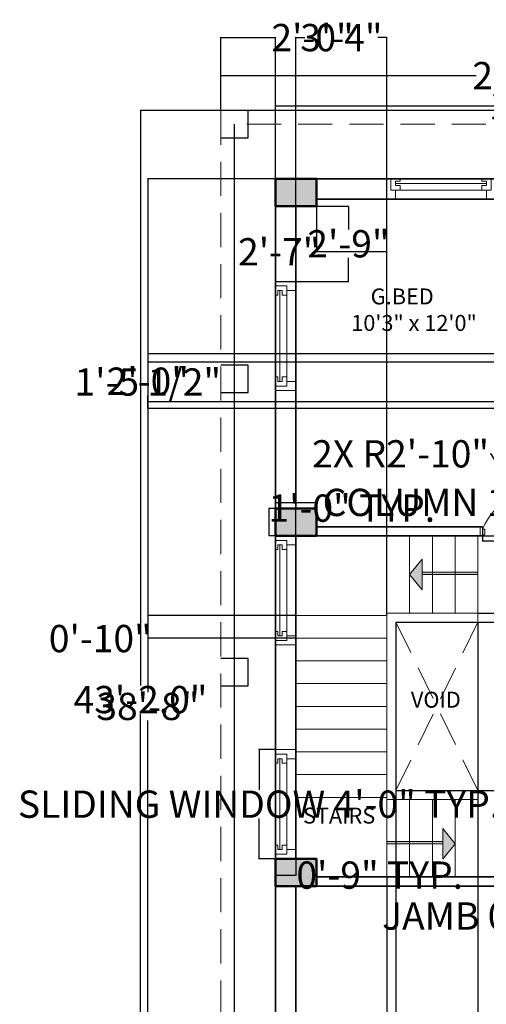
# Model space of a CAD drawing. Units: inches. Extents: x 1063 to 2718, y 423 to 1923.
# Tile 2 of 7: x 1063 to 1268, y 692 to 1125. Entities that reach past the tile are written whole.
import ezdxf

# ---------------------------------------------------------------- set-up
doc = ezdxf.new("R2010")
doc.units = ezdxf.units.IN
doc.header["$LTSCALE"] = 6
doc.header["$MEASUREMENT"] = 0
doc.linetypes.add('HIDDEN', pattern=[0.375, 0.25, -0.125])
for name, color, linetype, lineweight in [('A-ANNO-DIMS', 2, 'Continuous', 18), ('A-ANNO-SYMB', 4, 'Continuous', 18), ('A-ANNO-SYMB-PATT', 7, 'Continuous', 13), ('A-AREA-IDEN', 7, 'Continuous', 18), ('A-COLS', 7, 'Continuous', 50), ('A-COLS-PATT', 252, 'Continuous', 13), ('A-DOOR', 2, 'Continuous', 18), ('A-FLOR-STRS', 7, 'Continuous', 18), ('A-FLOR-STRS-HIDN', 7, 'HIDDEN', 13), ('A-GLAZ', 4, 'Continuous', 18), ('A-WALL', 7, 'Continuous', 35), ('C-PROP', 7, 'Continuous', 25), ('C-PROP-HIDN', 7, 'HIDDEN', 18)]:
    doc.layers.add(name, color=color, linetype=linetype, lineweight=lineweight)
doc.styles.get("Standard").update_dxf_attribs({"font": 'arial.ttf'})
doc.dimstyles.get("Standard").update_dxf_attribs({"dimtxt": 12, "dimasz": 0.18, "dimexe": 0.18, "dimexo": 0.0625, "dimgap": 0.09, "dimtad": 0, "dimtih": 1, "dimtoh": 1, "dimdec": 1, "dimzin": 0, "dimdsep": 46, "dimlunit": 3, "dimtxsty": 'Standard', "dimcen": 0.09, "dimadec": 0, "dimazin": 0, "dimtfac": 1, "dimtdec": 1, "dimtofl": 0, "dimtmove": 0, "dimatfit": 3, "dimfxl": 1, "dimtolj": 1, "dimtzin": 0, "dimarcsym": 0})

# ---------------------------------------------------------------- blocks, each defined once
blk = doc.blocks.new('*D1')
at = {"layer": 'A-ANNO-DIMS', "color": 0, "lineweight": -2, "ltscale": 6, "transparency": 16777216}
for p, q in [((1150.86, 1085.12), (1115.44, 1085.12)), ((1115.62, 1084.94), (1115.62, 832.34)), ((1115.62, 567.3), (1115.62, 819.9)), ((1150.86, 567.12), (1115.44, 567.12))]:
    blk.add_line(p, q, dxfattribs=at)
at = {"layer": 'A-ANNO-DIMS', "color": 0, "ltscale": 6, "transparency": 16777216}
for points in [[(1115.59, 1084.94), (1115.65, 1084.94), (1115.62, 1085.12)], [(1115.59, 567.3), (1115.65, 567.3), (1115.62, 567.12)]]:
    blk.add_solid(points, dxfattribs=at)
at = {"layer": 'Defpoints', "color": 0, "ltscale": 6, "transparency": 16777216}
for p in [(1115.62, 1085.12), (1150.93, 1085.12), (1150.93, 567.12)]:
    blk.add_point(p, dxfattribs=at)
at = {"layer": 'A-ANNO-DIMS', "color": 0, "ltscale": 6, "transparency": 16777216, "insert": (1115.62, 826.12), "char_height": 12, "attachment_point": 5}
blk.add_mtext('\\A1;43\'-2.0"', dxfattribs=at)
blk = doc.blocks.new('*D6')
at = {"layer": 'A-ANNO-DIMS', "color": 0, "lineweight": -2, "ltscale": 6, "transparency": 16777216}
for p, q in [((1150.93, 1085.18), (1150.93, 1100.66)), ((1151.11, 1100.48), (1263.13, 1100.48)), ((1430.75, 1100.48), (1318.72, 1100.48)), ((1430.93, 1085.18), (1430.93, 1100.66))]:
    blk.add_line(p, q, dxfattribs=at)
at = {"layer": 'A-ANNO-DIMS', "color": 0, "ltscale": 6, "transparency": 16777216}
for points in [[(1151.11, 1100.51), (1151.11, 1100.45), (1150.93, 1100.48)], [(1430.75, 1100.51), (1430.75, 1100.45), (1430.93, 1100.48)]]:
    blk.add_solid(points, dxfattribs=at)
at = {"layer": 'Defpoints', "color": 0, "ltscale": 6, "transparency": 16777216}
for p in [(1430.93, 1100.48), (1150.93, 1085.12), (1430.93, 1085.12)]:
    blk.add_point(p, dxfattribs=at)
at = {"layer": 'A-ANNO-DIMS', "color": 0, "ltscale": 6, "transparency": 16777216, "insert": (1290.93, 1100.48), "char_height": 12, "attachment_point": 5}
blk.add_mtext('\\A1;23\'-4.0"', dxfattribs=at)
blk = doc.blocks.new('WIN-48-SLIDING')
at = {"ltscale": 6}
for p, q in [((0, 9), (4, 9)), ((4, 9), (4, 5)), ((48, 9), (44, 9)), ((44, 9), (44, 5)), ((4, 5), (2, 5)), ((2, 5), (2, 0)), ((4, 5), (44, 5)), ((4, 5), (6, 5)), ((6, 5), (6, 3)), ((44, 5), (42, 5)), ((42, 5), (42, 3)), ((44, 5), (46, 5)), ((46, 5), (46, 0)), ((6, 3), (4, 3)), ((4, 3), (4, 1)), ((4, 2), (44, 2)), ((4, 1), (6, 1)), ((6, 1), (6, 0)), ((42, 3), (44, 3)), ((44, 1), (42, 1)), ((42, 1), (42, 0)), ((44, 3), (44, 1)), ((48, 0), (0, 0)), ((2, 0), (46, 0))]:
    blk.add_line(p, q, dxfattribs=at)
blk.add_lwpolyline([(48, 0), (48, 9), (0, 9), (0, 0)], dxfattribs=at)
blk = doc.blocks.new('DOOR-JAMB-4')
at = {"ltscale": 6}
for p, q in [((0, 0), (0, 4)), ((1, 4), (1, 3)), ((1, 3), (2, 3)), ((1.46, 0), (1.46, 0.33)), ((1.46, 0.33), (1.56, 0.33)), ((1.76, 0.53), (1.76, 0.69)), ((1.76, 0.69), (2, 0.69)), ((2, 3), (2, 0.69))]:
    blk.add_line(p, q, dxfattribs=at)
blk.add_arc((1.56, 0.53), 0.2, 270, 0, dxfattribs=at)
blk = doc.blocks.new('DOOR-LEAF-SINGLE-SWING')
at = {"ltscale": 6}
for p, q in [((34, 0), (13.24, 15)), ((35, 0.5), (13.9, 15.4))]:
    blk.add_line(p, q, dxfattribs=at)
blk.add_arc((31.02, -14.03), 34.04, 84.6951, 155.6613, dxfattribs=at)
blk = doc.blocks.new('COLUMN-18X12')
blk.add_lwpolyline([(0, 0), (18, 0), (18, 12), (0, 12)], close=True)
blk = doc.blocks.new('PIER-12X12-CORNER')
blk.add_lwpolyline([(0, 0), (12, 0), (12, 12)])
blk = doc.blocks.new('PIER-12X12-INLINE')
blk.add_lwpolyline([(0, 0), (12, 0), (12, 12), (0, 12)])
blk = doc.blocks.new('STAIR-DIRECTION-ARROW')
at = {"ltscale": 6}
for p, q in [((0, 6.77), (5.45, 13.53)), ((5.45, 13.53), (5.45, 6.77)), ((0, 6.77), (5.45, 0)), ((30, 7.77), (5.45, 7.77)), ((30, 6.77), (5.45, 6.77)), ((5.45, 0), (5.45, 6.77))]:
    blk.add_line(p, q, dxfattribs=at)
blk = doc.blocks.new('*D26')
at = {"layer": 'A-ANNO-DIMS', "color": 0, "lineweight": -2, "ltscale": 6, "transparency": 16777216}
for p, q in [((1174.93, 910.18), (1174.93, 913)), ((1175.11, 912.82), (1192.75, 912.82)), ((1192.93, 910.18), (1192.93, 913)), ((1192.93, 912.82), (1193.11, 912.82))]:
    blk.add_line(p, q, dxfattribs=at)
at = {"layer": 'A-ANNO-DIMS', "color": 0, "ltscale": 6, "transparency": 16777216}
for points in [[(1175.11, 912.85), (1175.11, 912.79), (1174.93, 912.82)], [(1192.75, 912.85), (1192.75, 912.79), (1192.93, 912.82)]]:
    blk.add_solid(points, dxfattribs=at)
at = {"layer": 'Defpoints', "color": 0, "ltscale": 6, "transparency": 16777216}
for p in [(1174.93, 910.12), (1192.93, 912.82), (1192.93, 910.12)]:
    blk.add_point(p, dxfattribs=at)
at = {"layer": 'A-ANNO-DIMS', "color": 0, "ltscale": 6, "transparency": 16777216, "insert": (1268.35, 912.82), "char_height": 12, "attachment_point": 5}
blk.add_mtext('\\A1;COLUMN 1\'-6" TYP.', dxfattribs=at)
blk = doc.blocks.new('*D27')
at = {"layer": 'A-ANNO-DIMS', "color": 0, "lineweight": -2, "ltscale": 6, "transparency": 16777216}
for p, q in [((1174.86, 910.12), (1172.05, 910.12)), ((1172.23, 910.12), (1172.23, 910.3)), ((1172.23, 910.3), (1172.41, 910.3)), ((1172.23, 898.3), (1172.23, 909.94)), ((1174.86, 898.12), (1172.05, 898.12))]:
    blk.add_line(p, q, dxfattribs=at)
at = {"layer": 'A-ANNO-DIMS', "color": 0, "ltscale": 6, "transparency": 16777216}
for points in [[(1172.2, 909.94), (1172.26, 909.94), (1172.23, 910.12)], [(1172.2, 898.3), (1172.26, 898.3), (1172.23, 898.12)]]:
    blk.add_solid(points, dxfattribs=at)
at = {"layer": 'Defpoints', "color": 0, "ltscale": 6, "transparency": 16777216}
for p in [(1172.23, 910.12), (1174.93, 910.12), (1174.93, 898.12)]:
    blk.add_point(p, dxfattribs=at)
at = {"layer": 'A-ANNO-DIMS', "color": 0, "ltscale": 6, "transparency": 16777216, "insert": (1208.5, 910.3), "char_height": 12, "attachment_point": 5}
blk.add_mtext('\\A1;1\'-0" TYP.', dxfattribs=at)
blk = doc.blocks.new('*D28')
at = {"layer": 'A-ANNO-DIMS', "color": 0, "lineweight": -2, "ltscale": 6, "transparency": 16777216}
for p, q in [((1174.86, 804.12), (1167.55, 804.12)), ((1167.73, 803.94), (1167.73, 786.42)), ((1167.73, 756.3), (1167.73, 773.82)), ((1174.86, 756.12), (1167.55, 756.12))]:
    blk.add_line(p, q, dxfattribs=at)
at = {"layer": 'A-ANNO-DIMS', "color": 0, "ltscale": 6, "transparency": 16777216}
for points in [[(1167.7, 803.94), (1167.76, 803.94), (1167.73, 804.12)], [(1167.7, 756.3), (1167.76, 756.3), (1167.73, 756.12)]]:
    blk.add_solid(points, dxfattribs=at)
at = {"layer": 'Defpoints', "color": 0, "ltscale": 6, "transparency": 16777216}
for p in [(1174.93, 804.12), (1167.73, 756.12), (1174.93, 756.12)]:
    blk.add_point(p, dxfattribs=at)
at = {"layer": 'A-ANNO-DIMS', "color": 0, "ltscale": 6, "transparency": 16777216, "insert": (1167.73, 780.12), "char_height": 12, "attachment_point": 5}
blk.add_mtext('\\A1;SLIDING WINDOW 4\'-0" TYP.', dxfattribs=at)
blk = doc.blocks.new('*D29')
at = {"layer": 'A-ANNO-DIMS', "color": 0, "lineweight": -2, "ltscale": 6, "transparency": 16777216}
for p, q in [((1174.93, 756.06), (1174.93, 748.74)), ((1183.93, 756.06), (1183.93, 748.74)), ((1175.11, 748.92), (1183.75, 748.92)), ((1183.93, 748.92), (1184.11, 748.92))]:
    blk.add_line(p, q, dxfattribs=at)
at = {"layer": 'A-ANNO-DIMS', "color": 0, "ltscale": 6, "transparency": 16777216}
for points in [[(1175.11, 748.95), (1175.11, 748.89), (1174.93, 748.92)], [(1183.75, 748.95), (1183.75, 748.89), (1183.93, 748.92)]]:
    blk.add_solid(points, dxfattribs=at)
at = {"layer": 'Defpoints', "color": 0, "ltscale": 6, "transparency": 16777216}
for p in [(1174.93, 756.12), (1183.93, 756.12), (1183.93, 748.92)]:
    blk.add_point(p, dxfattribs=at)
at = {"layer": 'A-ANNO-DIMS', "color": 0, "ltscale": 6, "transparency": 16777216, "insert": (1220.77, 748.92), "char_height": 12, "attachment_point": 5}
blk.add_mtext('\\A1;0\'-9" TYP.', dxfattribs=at)
blk = doc.blocks.new('*D32')
at = {"layer": 'A-ANNO-DIMS', "color": 0, "lineweight": -2, "ltscale": 6, "transparency": 16777216}
for p, q in [((1343.86, 735.12), (1343.15, 735.12)), ((1343.33, 734.94), (1343.33, 731.3)), ((1343.86, 731.12), (1343.15, 731.12)), ((1343.33, 730.94), (1343.15, 730.94)), ((1343.33, 731.12), (1343.33, 730.94))]:
    blk.add_line(p, q, dxfattribs=at)
at = {"layer": 'A-ANNO-DIMS', "color": 0, "ltscale": 6, "transparency": 16777216}
for points in [[(1343.3, 734.94), (1343.36, 734.94), (1343.33, 735.12)], [(1343.3, 731.3), (1343.36, 731.3), (1343.33, 731.12)]]:
    blk.add_solid(points, dxfattribs=at)
at = {"layer": 'Defpoints', "color": 0, "ltscale": 6, "transparency": 16777216}
for p in [(1343.93, 735.12), (1343.33, 731.12), (1343.93, 731.12)]:
    blk.add_point(p, dxfattribs=at)
at = {"layer": 'A-ANNO-DIMS', "color": 0, "ltscale": 6, "transparency": 16777216, "insert": (1281.68, 730.94), "char_height": 12, "attachment_point": 5}
blk.add_mtext('\\A1;JAMB 0\'-4" TYP.', dxfattribs=at)
blk = doc.blocks.new('*D42')
at = {"layer": 'A-ANNO-DIMS', "color": 0, "lineweight": -2, "ltscale": 6, "transparency": 16777216}
for p, q in [((1265.93, 901.06), (1265.93, 895.69)), ((1300.93, 901.06), (1300.93, 895.69)), ((1266.11, 895.87), (1300.75, 895.87)), ((1300.93, 895.87), (1301.11, 895.87))]:
    blk.add_line(p, q, dxfattribs=at)
at = {"layer": 'A-ANNO-DIMS', "color": 0, "ltscale": 6, "transparency": 16777216}
for points in [[(1266.11, 895.9), (1266.11, 895.84), (1265.93, 895.87)], [(1300.75, 895.9), (1300.75, 895.84), (1300.93, 895.87)]]:
    blk.add_solid(points, dxfattribs=at)
at = {"layer": 'Defpoints', "color": 0, "ltscale": 6, "transparency": 16777216}
for p in [(1265.93, 901.12), (1300.93, 901.12), (1300.93, 895.87)]:
    blk.add_point(p, dxfattribs=at)
at = {"layer": 'A-ANNO-DIMS', "color": 0, "ltscale": 6, "transparency": 16777216, "insert": (1398.77, 895.87), "char_height": 12, "attachment_point": 5}
blk.add_mtext('\\A1;SINGLE LEAF 2\'-11" TYP.', dxfattribs=at)
blk = doc.blocks.new('*D44')
at = {"layer": 'A-ANNO-DIMS', "color": 0, "lineweight": -2, "ltscale": 6, "transparency": 16777216}
for p, q in [((1174.93, 1055.18), (1174.93, 1087.4)), ((1175.11, 1087.22), (1271.29, 1087.22)), ((1407.75, 1087.22), (1311.56, 1087.22)), ((1407.93, 1055.18), (1407.93, 1087.4))]:
    blk.add_line(p, q, dxfattribs=at)
at = {"layer": 'A-ANNO-DIMS', "color": 0, "ltscale": 6, "transparency": 16777216}
for points in [[(1175.11, 1087.25), (1175.11, 1087.19), (1174.93, 1087.22)], [(1407.75, 1087.25), (1407.75, 1087.19), (1407.93, 1087.22)]]:
    blk.add_solid(points, dxfattribs=at)
at = {"layer": 'Defpoints', "color": 0, "ltscale": 6, "transparency": 16777216}
for p in [(1407.93, 1087.22), (1174.93, 1055.12), (1407.93, 1055.12)]:
    blk.add_point(p, dxfattribs=at)
at = {"layer": 'A-ANNO-DIMS', "color": 0, "ltscale": 6, "transparency": 16777216, "insert": (1291.43, 1087.22), "char_height": 12, "attachment_point": 5}
blk.add_mtext('\\A1;19\'-5"', dxfattribs=at)
blk = doc.blocks.new('*D45')
at = {"layer": 'A-ANNO-DIMS', "color": 0, "lineweight": -2, "ltscale": 6, "transparency": 16777216}
for p, q in [((1174.86, 1055.12), (1118.65, 1055.12)), ((1118.83, 1054.94), (1118.83, 829.34)), ((1118.83, 591.3), (1118.83, 816.9)), ((1174.86, 591.12), (1118.65, 591.12))]:
    blk.add_line(p, q, dxfattribs=at)
at = {"layer": 'A-ANNO-DIMS', "color": 0, "ltscale": 6, "transparency": 16777216}
for points in [[(1118.8, 1054.94), (1118.86, 1054.94), (1118.83, 1055.12)], [(1118.8, 591.3), (1118.86, 591.3), (1118.83, 591.12)]]:
    blk.add_solid(points, dxfattribs=at)
at = {"layer": 'Defpoints', "color": 0, "ltscale": 6, "transparency": 16777216}
for p in [(1118.83, 1055.12), (1174.93, 1055.12), (1174.93, 591.12)]:
    blk.add_point(p, dxfattribs=at)
at = {"layer": 'A-ANNO-DIMS', "color": 0, "ltscale": 6, "transparency": 16777216, "insert": (1118.83, 823.12), "char_height": 12, "attachment_point": 5}
blk.add_mtext('\\A1;38\'-8"', dxfattribs=at)
blk = doc.blocks.new('*D46')
at = {"layer": 'A-ANNO-DIMS', "color": 0, "lineweight": -2, "ltscale": 6, "transparency": 16777216}
for p, q in [((1150.93, 1085.18), (1150.93, 1117.4)), ((1151.11, 1117.22), (1174.75, 1117.22)), ((1174.93, 1055.18), (1174.93, 1117.4)), ((1174.93, 1117.22), (1175.11, 1117.22))]:
    blk.add_line(p, q, dxfattribs=at)
at = {"layer": 'A-ANNO-DIMS', "color": 0, "ltscale": 6, "transparency": 16777216}
for points in [[(1151.11, 1117.25), (1151.11, 1117.19), (1150.93, 1117.22)], [(1174.75, 1117.25), (1174.75, 1117.19), (1174.93, 1117.22)]]:
    blk.add_solid(points, dxfattribs=at)
at = {"layer": 'Defpoints', "color": 0, "ltscale": 6, "transparency": 16777216}
for p in [(1174.93, 1117.22), (1150.93, 1085.12), (1174.93, 1055.12)]:
    blk.add_point(p, dxfattribs=at)
at = {"layer": 'A-ANNO-DIMS', "color": 0, "ltscale": 6, "transparency": 16777216, "insert": (1191.25, 1117.22), "char_height": 12, "attachment_point": 5}
blk.add_mtext('\\A1;2\'-0"', dxfattribs=at)
blk = doc.blocks.new('*D50')
at = {"layer": 'A-ANNO-DIMS', "color": 0, "lineweight": -2, "ltscale": 6, "transparency": 16777216}
for p, q in [((1566.93, 731.06), (1566.93, 431.18)), ((1150.93, 567.06), (1150.93, 431.18)), ((1151.11, 431.36), (1338.23, 431.36)), ((1566.75, 431.36), (1379.62, 431.36))]:
    blk.add_line(p, q, dxfattribs=at)
at = {"layer": 'A-ANNO-DIMS', "color": 0, "ltscale": 6, "transparency": 16777216}
for points in [[(1151.11, 431.39), (1151.11, 431.33), (1150.93, 431.36)], [(1566.75, 431.39), (1566.75, 431.33), (1566.93, 431.36)]]:
    blk.add_solid(points, dxfattribs=at)
at = {"layer": 'Defpoints', "color": 0, "ltscale": 6, "transparency": 16777216}
for p in [(1566.93, 731.12), (1150.93, 567.12), (1566.93, 431.36)]:
    blk.add_point(p, dxfattribs=at)
at = {"layer": 'A-ANNO-DIMS', "color": 0, "ltscale": 6, "transparency": 16777216, "insert": (1358.93, 431.36), "char_height": 12, "attachment_point": 5}
blk.add_mtext('\\A1;34\'-8"', dxfattribs=at)
blk = doc.blocks.new('*D53')
at = {"layer": 'A-ANNO-DIMS', "color": 0, "lineweight": -2, "ltscale": 6, "transparency": 16777216}
for p, q in [((1183.93, 863.18), (1183.93, 1117.4)), ((1184.11, 1117.22), (1187.89, 1117.22)), ((1223.75, 1117.22), (1219.96, 1117.22)), ((1223.93, 863.18), (1223.93, 1117.4))]:
    blk.add_line(p, q, dxfattribs=at)
at = {"layer": 'A-ANNO-DIMS', "color": 0, "ltscale": 6, "transparency": 16777216}
for points in [[(1184.11, 1117.25), (1184.11, 1117.19), (1183.93, 1117.22)], [(1223.75, 1117.25), (1223.75, 1117.19), (1223.93, 1117.22)]]:
    blk.add_solid(points, dxfattribs=at)
at = {"layer": 'Defpoints', "color": 0, "ltscale": 6, "transparency": 16777216}
for p in [(1223.93, 1117.22), (1183.93, 863.12), (1223.93, 863.12)]:
    blk.add_point(p, dxfattribs=at)
at = {"layer": 'A-ANNO-DIMS', "color": 0, "ltscale": 6, "transparency": 16777216, "insert": (1203.93, 1117.22), "char_height": 12, "attachment_point": 5}
blk.add_mtext('\\A1;3\'-4"', dxfattribs=at)
blk = doc.blocks.new('*D54')
at = {"layer": 'A-ANNO-DIMS', "color": 0, "lineweight": -2, "ltscale": 6, "transparency": 16777216}
for p, q in [((1227.99, 860.12), (1599.21, 860.12)), ((1599.03, 859.94), (1599.03, 829.34)), ((1599.03, 786.3), (1599.03, 816.9)), ((1227.99, 786.12), (1599.21, 786.12))]:
    blk.add_line(p, q, dxfattribs=at)
at = {"layer": 'A-ANNO-DIMS', "color": 0, "ltscale": 6, "transparency": 16777216}
for points in [[(1599, 859.94), (1599.06, 859.94), (1599.03, 860.12)], [(1599, 786.3), (1599.06, 786.3), (1599.03, 786.12)]]:
    blk.add_solid(points, dxfattribs=at)
at = {"layer": 'Defpoints', "color": 0, "ltscale": 6, "transparency": 16777216}
for p in [(1227.93, 860.12), (1227.93, 786.12), (1599.03, 786.12)]:
    blk.add_point(p, dxfattribs=at)
at = {"layer": 'A-ANNO-DIMS', "color": 0, "ltscale": 6, "transparency": 16777216, "insert": (1599.03, 823.12), "char_height": 12, "attachment_point": 5}
blk.add_mtext('\\A1;6\'-2"', dxfattribs=at)
blk = doc.blocks.new('*D55')
at = {"layer": 'A-ANNO-DIMS', "color": 0, "lineweight": -2, "ltscale": 6, "transparency": 16777216}
for p, q in [((1227.93, 860.06), (1227.93, 431.18)), ((1263.93, 860.06), (1263.93, 431.18)), ((1228.11, 431.36), (1229.89, 431.36)), ((1263.75, 431.36), (1261.96, 431.36))]:
    blk.add_line(p, q, dxfattribs=at)
at = {"layer": 'A-ANNO-DIMS', "color": 0, "ltscale": 6, "transparency": 16777216}
for points in [[(1228.11, 431.39), (1228.11, 431.33), (1227.93, 431.36)], [(1263.75, 431.39), (1263.75, 431.33), (1263.93, 431.36)]]:
    blk.add_solid(points, dxfattribs=at)
at = {"layer": 'Defpoints', "color": 0, "ltscale": 6, "transparency": 16777216}
for p in [(1227.93, 860.12), (1263.93, 860.12), (1263.93, 431.36)]:
    blk.add_point(p, dxfattribs=at)
at = {"layer": 'A-ANNO-DIMS', "color": 0, "ltscale": 6, "transparency": 16777216, "insert": (1245.93, 431.36), "char_height": 12, "attachment_point": 5}
blk.add_mtext('\\A1;3\'-0"', dxfattribs=at)
blk = doc.blocks.new('*D56')
at = {"layer": 'A-ANNO-DIMS', "color": 0, "lineweight": -2, "ltscale": 6, "transparency": 16777216}
for p, q in [((1183.86, 863.12), (1118.65, 863.12)), ((1118.83, 862.94), (1118.83, 853.3)), ((1183.86, 853.12), (1118.65, 853.12)), ((1118.83, 853.12), (1118.83, 852.94)), ((1118.83, 852.94), (1118.65, 852.94))]:
    blk.add_line(p, q, dxfattribs=at)
at = {"layer": 'A-ANNO-DIMS', "color": 0, "ltscale": 6, "transparency": 16777216}
for points in [[(1118.8, 862.94), (1118.86, 862.94), (1118.83, 863.12)], [(1118.8, 853.3), (1118.86, 853.3), (1118.83, 853.12)]]:
    blk.add_solid(points, dxfattribs=at)
at = {"layer": 'Defpoints', "color": 0, "ltscale": 6, "transparency": 16777216}
for p in [(1183.93, 863.12), (1118.83, 853.12), (1183.93, 853.12)]:
    blk.add_point(p, dxfattribs=at)
at = {"layer": 'A-ANNO-DIMS', "color": 0, "ltscale": 6, "transparency": 16777216, "insert": (1097.94, 852.94), "char_height": 12, "attachment_point": 5}
blk.add_mtext('\\A1;0\'-10"', dxfattribs=at)
blk = doc.blocks.new('*D57')
at = {"layer": 'A-ANNO-DIMS', "color": 0, "lineweight": -2, "ltscale": 6, "transparency": 16777216}
for p, q in [((1263.99, 898.12), (1296.21, 898.12)), ((1296.03, 897.94), (1296.03, 887.34)), ((1296.03, 864.3), (1296.03, 874.9)), ((1263.99, 864.12), (1296.21, 864.12))]:
    blk.add_line(p, q, dxfattribs=at)
at = {"layer": 'A-ANNO-DIMS', "color": 0, "ltscale": 6, "transparency": 16777216}
for points in [[(1296, 897.94), (1296.06, 897.94), (1296.03, 898.12)], [(1296, 864.3), (1296.06, 864.3), (1296.03, 864.12)]]:
    blk.add_solid(points, dxfattribs=at)
at = {"layer": 'Defpoints', "color": 0, "ltscale": 6, "transparency": 16777216}
for p in [(1263.93, 898.12), (1263.93, 864.12), (1296.03, 864.12)]:
    blk.add_point(p, dxfattribs=at)
at = {"layer": 'A-ANNO-DIMS', "color": 0, "ltscale": 6, "transparency": 16777216, "insert": (1296.03, 881.12), "char_height": 12, "attachment_point": 5}
blk.add_mtext('\\A1;2\'-10"', dxfattribs=at)
blk = doc.blocks.new('*D58')
at = {"layer": 'A-ANNO-DIMS', "color": 0, "lineweight": -2, "ltscale": 6, "transparency": 16777216}
for p, q in [((1223.93, 748.06), (1223.93, 431.18)), ((1263.93, 748.06), (1263.93, 431.18)), ((1224.11, 431.36), (1227.89, 431.36)), ((1263.75, 431.36), (1259.96, 431.36))]:
    blk.add_line(p, q, dxfattribs=at)
at = {"layer": 'A-ANNO-DIMS', "color": 0, "ltscale": 6, "transparency": 16777216}
for points in [[(1224.11, 431.39), (1224.11, 431.33), (1223.93, 431.36)], [(1263.75, 431.39), (1263.75, 431.33), (1263.93, 431.36)]]:
    blk.add_solid(points, dxfattribs=at)
at = {"layer": 'Defpoints', "color": 0, "ltscale": 6, "transparency": 16777216}
for p in [(1223.93, 748.12), (1263.93, 748.12), (1263.93, 431.36)]:
    blk.add_point(p, dxfattribs=at)
at = {"layer": 'A-ANNO-DIMS', "color": 0, "ltscale": 6, "transparency": 16777216, "insert": (1243.93, 431.36), "char_height": 12, "attachment_point": 5}
blk.add_mtext('\\A1;3\'-4"', dxfattribs=at)
blk = doc.blocks.new('*D59')
at = {"layer": 'A-ANNO-DIMS', "color": 0, "lineweight": -2, "ltscale": 6, "transparency": 16777216}
for p, q in [((1310.86, 978.12), (1118.65, 978.12)), ((1118.83, 977.94), (1118.83, 972.34)), ((1118.83, 954.3), (1118.83, 959.9)), ((1310.86, 954.12), (1118.65, 954.12))]:
    blk.add_line(p, q, dxfattribs=at)
at = {"layer": 'A-ANNO-DIMS', "color": 0, "ltscale": 6, "transparency": 16777216}
for points in [[(1118.8, 977.94), (1118.86, 977.94), (1118.83, 978.12)], [(1118.8, 954.3), (1118.86, 954.3), (1118.83, 954.12)]]:
    blk.add_solid(points, dxfattribs=at)
at = {"layer": 'Defpoints', "color": 0, "ltscale": 6, "transparency": 16777216}
for p in [(1310.93, 978.12), (1118.83, 954.12), (1310.93, 954.12)]:
    blk.add_point(p, dxfattribs=at)
at = {"layer": 'A-ANNO-DIMS', "color": 0, "ltscale": 6, "transparency": 16777216, "insert": (1118.83, 966.12), "char_height": 12, "attachment_point": 5}
blk.add_mtext('\\A1;2\'-0"', dxfattribs=at)
blk = doc.blocks.new('*D61')
at = {"layer": 'A-ANNO-DIMS', "color": 0, "lineweight": -2, "ltscale": 6, "transparency": 16777216}
for p, q in [((1321.15, 974.55), (1118.65, 974.55)), ((1118.83, 974.37), (1118.83, 972.07)), ((1321.15, 956.99), (1118.65, 956.99)), ((1118.83, 957.17), (1118.83, 959.48))]:
    blk.add_line(p, q, dxfattribs=at)
at = {"layer": 'A-ANNO-DIMS', "color": 0, "ltscale": 6, "transparency": 16777216}
for points in [[(1118.8, 974.37), (1118.86, 974.37), (1118.83, 974.55)], [(1118.8, 957.17), (1118.86, 957.17), (1118.83, 956.99)]]:
    blk.add_solid(points, dxfattribs=at)
at = {"layer": 'Defpoints', "color": 0, "ltscale": 6, "transparency": 16777216}
for p in [(1118.83, 974.55), (1321.21, 974.55), (1321.21, 956.99)]:
    blk.add_point(p, dxfattribs=at)
at = {"layer": 'A-ANNO-DIMS', "color": 0, "ltscale": 6, "transparency": 16777216, "insert": (1118.83, 965.77), "char_height": 12, "attachment_point": 5}
blk.add_mtext('\\A1;1\'-5 1/2"', dxfattribs=at)
blk = doc.blocks.new('*D66')
at = {"layer": 'A-ANNO-DIMS', "color": 0, "lineweight": -2, "ltscale": 6, "transparency": 16777216}
for p, q in [((1192.93, 1055.06), (1192.93, 1022.84)), ((1223.72, 1055.06), (1223.72, 1022.84)), ((1192.93, 1023.02), (1192.75, 1023.02)), ((1223.54, 1023.02), (1193.11, 1023.02))]:
    blk.add_line(p, q, dxfattribs=at)
at = {"layer": 'A-ANNO-DIMS', "color": 0, "ltscale": 6, "transparency": 16777216}
for points in [[(1193.11, 1023.05), (1193.11, 1022.99), (1192.93, 1023.02)], [(1223.54, 1023.05), (1223.54, 1022.99), (1223.72, 1023.02)]]:
    blk.add_solid(points, dxfattribs=at)
at = {"layer": 'Defpoints', "color": 0, "ltscale": 6, "transparency": 16777216}
for p in [(1192.93, 1055.12), (1223.72, 1055.12), (1192.93, 1023.02)]:
    blk.add_point(p, dxfattribs=at)
at = {"layer": 'A-ANNO-DIMS', "color": 0, "ltscale": 6, "transparency": 16777216, "insert": (1176.6, 1023.02), "char_height": 12, "attachment_point": 5}
blk.add_mtext('\\A1;2\'-7"', dxfattribs=at)
blk = doc.blocks.new('*D67')
at = {"layer": 'A-ANNO-DIMS', "color": 0, "lineweight": -2, "ltscale": 6, "transparency": 16777216}
for p, q in [((1174.99, 1043.12), (1207.21, 1043.12)), ((1207.03, 1042.94), (1207.03, 1032.78)), ((1207.03, 1010.18), (1207.03, 1020.34)), ((1174.99, 1010), (1207.21, 1010))]:
    blk.add_line(p, q, dxfattribs=at)
at = {"layer": 'A-ANNO-DIMS', "color": 0, "ltscale": 6, "transparency": 16777216}
for points in [[(1207, 1042.94), (1207.06, 1042.94), (1207.03, 1043.12)], [(1207, 1010.18), (1207.06, 1010.18), (1207.03, 1010)]]:
    blk.add_solid(points, dxfattribs=at)
at = {"layer": 'Defpoints', "color": 0, "ltscale": 6, "transparency": 16777216}
for p in [(1174.93, 1043.12), (1174.93, 1010), (1207.03, 1010)]:
    blk.add_point(p, dxfattribs=at)
at = {"layer": 'A-ANNO-DIMS', "color": 0, "ltscale": 6, "transparency": 16777216, "insert": (1207.03, 1026.56), "char_height": 12, "attachment_point": 5}
blk.add_mtext('\\A1;2\'-9"', dxfattribs=at)
blk = doc.blocks.new('*D73')
at = {"layer": 'A-ANNO-DIMS', "color": 0, "lineweight": -2, "ltscale": 6, "transparency": 16777216}
for p, q in [((1269.38, 934.18), (1269.56, 934.18)), ((1269.56, 934.18), (1279.74, 916.67)), ((1296.85, 887.09), (1297.03, 887.09)), ((1296.94, 887), (1296.94, 887.18))]:
    blk.add_line(p, q, dxfattribs=at)
at = {"layer": 'A-ANNO-DIMS', "color": 0, "ltscale": 6, "transparency": 16777216}
blk.add_solid([(1279.77, 916.69), (1279.71, 916.66), (1279.83, 916.52)], dxfattribs=at)
at = {"layer": 'Defpoints', "color": 0, "ltscale": 6, "transparency": 16777216}
for p in [(1279.83, 916.52), (1296.94, 887.09)]:
    blk.add_point(p, dxfattribs=at)
at = {"layer": 'A-ANNO-DIMS', "color": 0, "ltscale": 6, "transparency": 16777216, "insert": (1229.94, 934.18), "char_height": 12, "attachment_point": 5}
blk.add_mtext('\\A1;2X R2\'-10"', dxfattribs=at)

msp = doc.modelspace()

# ---------------------------------------------------------------- hatches: boundary and pattern name
at = {"layer": 'A-ANNO-SYMB-PATT', "ltscale": 6}
h = msp.add_hatch(color=256, dxfattribs=at)
h.dxf.hatch_style = 1
h.paths.add_polyline_path([(1248.47, 769.4), (1248.47, 762.63), (1248.47, 755.87), (1253.93, 762.63)])
h.paths.add_polyline_path([(1248.47, 763.63), (1243.93, 763.63), (1243.93, 762.63), (1248.47, 762.63)])
h.paths.add_polyline_path([(1243.93, 763.63), (1233.93, 763.63), (1233.93, 762.63), (1243.93, 762.63)])
h.paths.add_polyline_path([(1233.93, 763.63), (1223.93, 763.63), (1223.93, 762.63), (1233.93, 762.63)])
h.paths.add_polyline_path([(1263.93, 882.12), (1253.93, 882.12), (1253.93, 881.12), (1263.93, 881.12)])
h.paths.add_polyline_path([(1253.93, 882.12), (1243.93, 882.12), (1243.93, 881.12), (1253.93, 881.12)])
h.paths.add_polyline_path([(1243.93, 882.12), (1239.38, 882.12), (1239.38, 881.12), (1243.93, 881.12)])
h.paths.add_polyline_path([(1239.38, 881.12), (1239.38, 882.12), (1239.38, 887.88), (1233.93, 881.12), (1239.38, 874.35)])
at = {"layer": 'A-COLS-PATT', "ltscale": 6}
h = msp.add_hatch(color=256, dxfattribs=at)
h.dxf.hatch_style = 1
h.paths.add_polyline_path([(1192.93, 603.12), (1174.93, 603.12), (1174.93, 591.12), (1192.93, 591.12)])
h.paths.add_polyline_path([(1407.93, 603.12), (1389.93, 603.12), (1389.93, 591.12), (1407.93, 591.12)])
h.paths.add_polyline_path([(1192.93, 756.12), (1174.93, 756.12), (1174.93, 744.12), (1192.93, 744.12)])
h.paths.add_polyline_path([(1407.93, 761.11), (1389.93, 761.11), (1389.93, 749.11), (1407.93, 749.11)])
h.paths.add_polyline_path([(1455.93, 761.11), (1437.93, 761.11), (1437.93, 749.11), (1455.93, 749.11)])
h.paths.add_polyline_path([(1455.93, 910.12), (1437.93, 910.12), (1437.93, 898.12), (1455.93, 898.12)])
h.paths.add_polyline_path([(1407.93, 910.12), (1389.93, 910.12), (1389.93, 898.12), (1407.93, 898.12)])
h.paths.add_polyline_path([(1192.93, 910.12), (1174.93, 910.12), (1174.93, 898.12), (1192.93, 898.12)])
h.paths.add_polyline_path([(1192.93, 1055.12), (1174.93, 1055.12), (1174.93, 1043.12), (1192.93, 1043.12)])
h.paths.add_polyline_path([(1407.93, 1055.12), (1389.93, 1055.12), (1389.93, 1043.12), (1407.93, 1043.12)])

# ---------------------------------------------------------------- linework, layer by layer
at = {"layer": 'A-FLOR-STRS'}
for p, q in [((1223.93, 898.12), (1223.93, 748.12)), ((1233.93, 864.12), (1233.93, 898.12)), ((1243.93, 864.12), (1243.93, 898.12)), ((1253.93, 864.12), (1253.93, 898.12)), ((1223.93, 863.12), (1183.93, 863.12)), ((1263.93, 864.12), (1223.93, 864.12)), ((1227.93, 860.12), (1227.93, 786.12)), ((1263.93, 860.12), (1227.93, 860.12)), ((1223.93, 853.12), (1183.93, 853.12)), ((1223.93, 843.12), (1183.93, 843.12)), ((1223.93, 833.12), (1183.93, 833.12)), ((1223.93, 823.12), (1183.93, 823.12)), ((1223.93, 813.12), (1183.93, 813.12)), ((1223.93, 803.12), (1183.93, 803.12)), ((1223.93, 793.12), (1183.93, 793.12)), ((1263.93, 786.12), (1227.93, 786.12)), ((1223.93, 783.12), (1183.93, 783.12)), ((1263.93, 782.12), (1223.93, 782.12)), ((1233.93, 748.12), (1233.93, 782.12)), ((1243.93, 748.12), (1243.93, 782.12)), ((1253.93, 748.12), (1253.93, 782.12))]:
    msp.add_line(p, q, dxfattribs=at)
at = {"layer": 'A-FLOR-STRS', "ltscale": 6}
for p, q in [((1263.93, 898.12), (1263.93, 864.12)), ((1263.93, 782.12), (1263.93, 748.12))]:
    msp.add_line(p, q, dxfattribs=at)
at = {"layer": 'A-FLOR-STRS-HIDN', "ltscale": 10}
for p, q in [((1263.93, 898.12), (1263.93, 748.12)), ((1263.93, 786.12), (1227.93, 860.12)), ((1263.93, 860.12), (1227.93, 786.12))]:
    msp.add_line(p, q, dxfattribs=at)
at = {"layer": 'A-WALL'}
for p, q in [((1407.93, 1055.12), (1174.93, 1055.12)), ((1306.93, 1046.12), (1192.93, 1046.12)), ((1183.93, 1043.12), (1183.93, 910.12)), ((1265.93, 902.12), (1192.93, 902.12)), ((1266.39, 898.12), (1183.93, 898.12)), ((1310.93, 748.12), (1192.93, 748.12)), ((1306.93, 744.12), (1183.93, 744.12))]:
    msp.add_line(p, q, dxfattribs=at)
at = {"layer": 'A-WALL', "ltscale": 6}
for p, q in [((1174.93, 1055.12), (1174.93, 591.12)), ((1183.93, 898.12), (1183.93, 756.12)), ((1183.93, 744.12), (1183.93, 603.12))]:
    msp.add_line(p, q, dxfattribs=at)
at = {"layer": 'C-PROP'}
for p, q in [((1430.93, 1085.12), (1150.93, 1085.12)), ((1156.93, 567.12), (1156.93, 1079.12))]:
    msp.add_line(p, q, dxfattribs=at)
at = {"layer": 'C-PROP-HIDN', "ltscale": 10}
for p, q in [((1150.93, 1085.12), (1150.93, 567.12)), ((1424.93, 1079.12), (1156.93, 1079.12))]:
    msp.add_line(p, q, dxfattribs=at)

# ---------------------------------------------------------------- block references
at = {"layer": 'A-ANNO-SYMB'}
msp.add_blockref('STAIR-DIRECTION-ARROW', (1233.93, 874.35), dxfattribs=at)
at = {"layer": 'A-ANNO-SYMB', "extrusion": (0, 0, -1), "zscale": -1}
msp.add_blockref('STAIR-DIRECTION-ARROW', (-1253.93, 755.87), dxfattribs=at)
at = {"layer": 'A-COLS'}
for p in [(1174.93, 1043.12), (1174.93, 898.12), (1174.93, 744.12)]:
    msp.add_blockref('COLUMN-18X12', p, dxfattribs=at)
at = {"layer": 'A-DOOR'}
for name, p in [('DOOR-LEAF-SINGLE-SWING', (1265.93, 901.12)), ('DOOR-JAMB-4', (1264.93, 898.12))]:
    msp.add_blockref(name, p, dxfattribs=at)
at = {"layer": 'A-GLAZ'}
for p, rotation in [((1271.72, 1055.12), 180), ((1174.93, 1010), 269.9999999999954), ((1174.93, 898.12), 269.9999999999978), ((1174.93, 804.12), 269.9999999999981)]:
    msp.add_blockref('WIN-48-SLIDING', p, dxfattribs=dict(at, rotation=rotation))
at = {"layer": 'C-PROP'}
for name, p in [('PIER-12X12-CORNER', (1150.93, 1073.12)), ('PIER-12X12-INLINE', (1150.93, 961.12)), ('PIER-12X12-INLINE', (1150.93, 832.12))]:
    msp.add_blockref(name, p, dxfattribs=at)

# ---------------------------------------------------------------- texts
at = {"layer": 'A-AREA-IDEN', "ltscale": 6, "char_height": 7, "attachment_point": 1}
for s, insert in [('    G.BED\\P10\'3" x 12\'0"', (1208.26, 1006.9)), ('VOID', (1234.47, 829.56)), ('STAIRS', (1187.04, 778.59))]:
    msp.add_mtext_dynamic_manual_height_columns(s, width=175.2385, gutter_width=1, heights=[0], dxfattribs=dict(at, insert=insert))

# ---------------------------------------------------------------- dimensions: what is measured, and where the dimension line sits
at = {"layer": 'A-ANNO-DIMS', "ltscale": 6}
for base, p1, p2, override, picture, middle in [((1174.93, 1117.22), (1150.93, 1085.12), (1174.93, 1055.12), {"dimdec": 1, "dimlfac": 1, "dimrnd": 0, "dimzin": 1, "dimdsep": 46, "dimlunit": 4, "dimfrac": 2}, '*D46', (1191.25, 1117.22)), ((1223.93, 1117.22), (1183.93, 863.12), (1223.93, 863.12), {"dimdec": 1, "dimlfac": 1, "dimrnd": 0, "dimzin": 1, "dimdsep": 46, "dimlunit": 4, "dimfrac": 2}, '*D53', (1203.93, 1117.22)), ((1430.93, 1100.48), (1150.93, 1085.12), (1430.93, 1085.12), {"dimclrd": 0, "dimclre": 0, "dimclrt": 0}, '*D6', (1290.93, 1100.48)), ((1407.93, 1087.22), (1174.93, 1055.12), (1407.93, 1055.12), {"dimdec": 1, "dimlfac": 1, "dimrnd": 0, "dimzin": 1, "dimdsep": 46, "dimlunit": 4, "dimfrac": 2}, '*D44', (1291.43, 1087.22)), ((1263.93, 431.36), (1227.93, 860.12), (1263.93, 860.12), {"dimdec": 1, "dimlfac": 1, "dimrnd": 0, "dimzin": 1, "dimdsep": 46, "dimlunit": 4, "dimfrac": 2}, '*D55', (1245.93, 431.36)), ((1263.93, 431.36), (1223.93, 748.12), (1263.93, 748.12), {"dimdec": 1, "dimlfac": 1, "dimrnd": 0, "dimzin": 1, "dimdsep": 46, "dimlunit": 4, "dimfrac": 2}, '*D58', (1243.93, 431.36)), ((1566.93, 431.36), (1150.93, 567.12), (1566.93, 731.12), {"dimdec": 1, "dimlfac": 1, "dimrnd": 0, "dimzin": 1, "dimdsep": 46, "dimlunit": 4, "dimfrac": 2}, '*D50', (1358.93, 431.36))]:
    dim = msp.add_linear_dim(base=base, p1=p1, p2=p2, dimstyle='Standard', override=override, dxfattribs=at)
    dim.commit()
    dim.dimension.update_dxf_attribs({"geometry": picture, "text_midpoint": middle})
for base, p1, p2, angle, override, picture, middle in [((1115.62, 1085.12), (1150.93, 567.12), (1150.93, 1085.12), 90, {"dimclrd": 0, "dimclre": 0, "dimclrt": 0}, '*D1', (1115.62, 826.12)), ((1118.83, 1055.12), (1174.93, 591.12), (1174.93, 1055.12), 90, {"dimdec": 1, "dimlfac": 1, "dimrnd": 0, "dimzin": 1, "dimdsep": 46, "dimlunit": 4, "dimfrac": 2}, '*D45', (1118.83, 823.12)), ((1192.93, 1023.02), (1223.72, 1055.12), (1192.93, 1055.12), 180, {"dimdec": 1, "dimlfac": 1, "dimrnd": 0, "dimzin": 1, "dimdsep": 46, "dimlunit": 4, "dimfrac": 2}, '*D66', (1176.6, 1023.02)), ((1207.03, 1010), (1174.93, 1043.12), (1174.93, 1010), 270, {"dimdec": 1, "dimlfac": 1, "dimrnd": 0, "dimzin": 1, "dimdsep": 46, "dimlunit": 4, "dimfrac": 2}, '*D67', (1207.03, 1026.56)), ((1118.83, 974.55), (1321.21, 956.99), (1321.21, 974.55), 90, {"dimdec": 1, "dimlfac": 1, "dimrnd": 0, "dimzin": 1, "dimdsep": 46, "dimlunit": 4, "dimfrac": 2}, '*D61', (1118.83, 965.77)), ((1118.83, 954.12), (1310.93, 978.12), (1310.93, 954.12), 90, {"dimdec": 1, "dimlfac": 1, "dimrnd": 0, "dimzin": 1, "dimdsep": 46, "dimlunit": 4, "dimfrac": 2}, '*D59', (1118.83, 966.12)), ((1296.03, 864.12), (1263.93, 898.12), (1263.93, 864.12), 270, {"dimdec": 1, "dimlfac": 1, "dimrnd": 0, "dimzin": 1, "dimdsep": 46, "dimlunit": 4, "dimfrac": 2}, '*D57', (1296.03, 881.12)), ((1118.83, 853.12), (1183.93, 863.12), (1183.93, 853.12), 90, {"dimdec": 1, "dimlfac": 1, "dimrnd": 0, "dimzin": 1, "dimdsep": 46, "dimlunit": 4, "dimfrac": 2}, '*D56', (1097.94, 852.94)), ((1599.03, 786.12), (1227.93, 860.12), (1227.93, 786.12), 90, {"dimdec": 1, "dimlfac": 1, "dimrnd": 0, "dimzin": 1, "dimdsep": 46, "dimlunit": 4, "dimfrac": 2}, '*D54', (1599.03, 823.12))]:
    dim = msp.add_linear_dim(base=base, p1=p1, p2=p2, angle=angle, dimstyle='Standard', override=override, dxfattribs=at)
    dim.commit()
    dim.dimension.update_dxf_attribs({"geometry": picture, "text_midpoint": middle})
dim = msp.add_radius_dim(center=(1296.94, 887.09), mpoint=(1279.83, 916.52), text='2X <>', dimstyle='Standard', override={"dimdec": 1, "dimlfac": 1, "dimrnd": 0, "dimzin": 1, "dimdsep": 46, "dimlunit": 4, "dimfrac": 2}, dxfattribs=at)
dim.commit()
dim.dimension.update_dxf_attribs({"geometry": '*D73', "text_midpoint": (1229.94, 934.18), "dimtype": 164})
for base, p1, p2, text, picture, middle in [((1192.93, 912.82), (1174.93, 910.12), (1192.93, 910.12), 'COLUMN <> TYP.', '*D26', (1268.35, 912.82)), ((1300.93, 895.87), (1265.93, 901.12), (1300.93, 901.12), 'SINGLE LEAF <> TYP.', '*D42', (1398.77, 895.87)), ((1183.93, 748.92), (1174.93, 756.12), (1183.93, 756.12), '<> TYP.', '*D29', (1220.77, 748.92))]:
    dim = msp.add_linear_dim(base=base, p1=p1, p2=p2, text=text, dimstyle='Standard', override={"dimdec": 1, "dimlfac": 1, "dimrnd": 0, "dimzin": 1, "dimdsep": 46, "dimlunit": 4, "dimfrac": 2}, dxfattribs=at)
    dim.commit()
    dim.dimension.update_dxf_attribs({"geometry": picture, "text_midpoint": middle})
for base, p1, p2, angle, text, picture, middle in [((1172.23, 910.12), (1174.93, 898.12), (1174.93, 910.12), 90, '<> TYP.', '*D27', (1208.5, 910.3)), ((1167.73, 756.12), (1174.93, 804.12), (1174.93, 756.12), 270, 'SLIDING WINDOW <> TYP.', '*D28', (1167.73, 780.12)), ((1343.33, 731.12), (1343.93, 735.12), (1343.93, 731.12), 270, 'JAMB <> TYP.', '*D32', (1281.68, 730.94))]:
    dim = msp.add_linear_dim(base=base, p1=p1, p2=p2, angle=angle, text=text, dimstyle='Standard', override={"dimdec": 1, "dimlfac": 1, "dimrnd": 0, "dimzin": 1, "dimdsep": 46, "dimlunit": 4, "dimfrac": 2}, dxfattribs=at)
    dim.commit()
    dim.dimension.update_dxf_attribs({"geometry": picture, "text_midpoint": middle})

doc.saveas('drawing.dxf')
